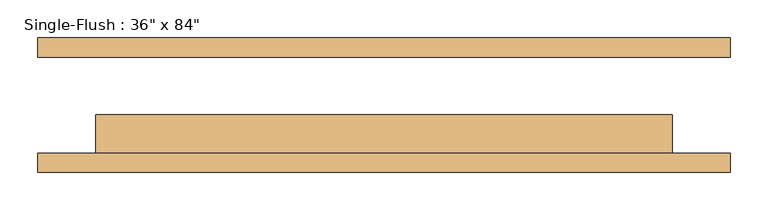
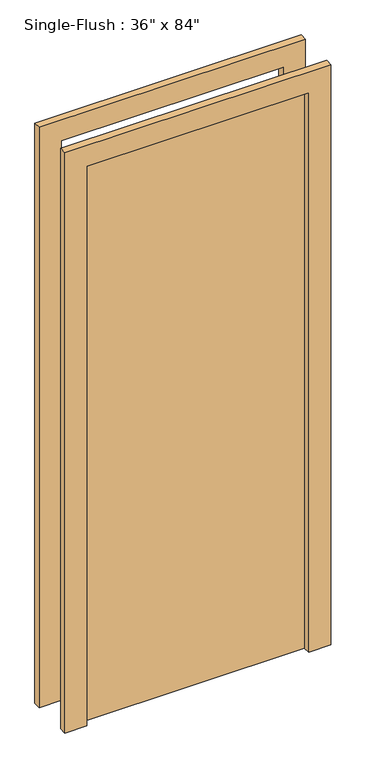
"""IFC4 building model written with IfcOpenShell, lengths in millimetres: door geometry."""

from ifc_helpers import new_model, si_unit, frame, origin, origin_with_axes, place, context, project, spatial, polyline, outline, extrude, source, transform, mapped, element, save


def door_e00f436c(model_context):
    return source(origin(), model_context, "Body", "SweptSolid", [
        extrude(outline(polyline([(2108.2, -457.2), (0.0, -457.2), (0.0, -381.0), (2032.0, -381.0), (2032.0, 381.0), (0.0, 381.0), (0.0, 457.2), (2108.2, 457.2), (2108.2, -457.2)])), frame((0.0, -88.9, 0.0), z_axis=(0.0, 1.0, 0.0), x_axis=(0.0, 0.0, 1.0)), (0.0, 0.0, 1.0), 25.4),
        extrude(outline(polyline([(2108.2, 457.2), (2108.2, -457.2), (0.0, -457.2), (0.0, -381.0), (2032.0, -381.0), (2032.0, 381.0), (0.0, 381.0), (0.0, 457.2), (2108.2, 457.2)])), frame((0.0, 63.5, 0.0), z_axis=(0.0, 1.0, 0.0), x_axis=(0.0, 0.0, 1.0)), (0.0, 0.0, 1.0), 25.4),
        extrude(outline(polyline([(381.0, -12.7), (381.0, -63.5), (-381.0, -63.5), (-381.0, -12.7), (381.0, -12.7)])), origin_with_axes(), (0.0, 0.0, 1.0), 2032.0),
    ])


if __name__ == "__main__":
    model = new_model("IFC4")
    model_context = context("Model", 3, world=origin())
    ifc_project = project(units=[si_unit("LENGTHUNIT", "METRE", prefix="MILLI")], contexts=[model_context])
    site = spatial("IfcSite", under=ifc_project)
    building = spatial("IfcBuilding", under=site)
    placement = place(None, origin())
    door_shape = door_e00f436c(model_context)
    element("IfcDoor", 1, ObjectType="Single-Flush : 36\" x 84\"", at=placement, inside=building, context=model_context, shape_type="MappedRepresentation", body=[
        mapped(door_shape, transform((0.0, 0.0, 0.0), x_axis=(1.0, 0.0, 0.0), y_axis=(0.0, 1.0, 0.0), z_axis=(0.0, 0.0, 1.0))),
    ])
    save(model, "model.ifc")

# Revit data of these elements
# Type "Single-Flush : 36\" x 84\""
#   Type Mark = "1"
#   Construction Type Id = "MDOOR"
#   Assembly Code = "C1020"
#   Analytic Construction = "Metal"
#   Thickness = 0' - 2"
#   Heat Transfer Coefficient (U) = 0.651978 BTU/(h·ft²·°F)
#   Height = 6' - 8"
#   Trim Projection Ext = 0' - 1"
#   Trim Projection Int = 0' - 1"
#   Trim Width = 0' - 3"
#   Width = 2' - 6"
#   Define Thermal Properties by = 1
#   Define Thermal Properties by = 1
#   Door Material = Door - Panel
#   Frame Material = Door - Frame
#   Visual Light Transmittance = 0
#   Solar Heat Gain Coefficient = 0
#   Function = (empty or 0)
#   Wall Closure = (empty or 0)
# Element 1 (IfcDoor, "Single-Flush : 36\" x 84\"")
#   Materials on its faces: "Door - Frame", "Door - Panel"
# Materials
#   "Door - Panel": class "Wood", colour RGB 210 159 95, transparency 0, Cost = 0
#   "Door - Frame": colour RGB 118 70 51, transparency 0, Cost = 0
